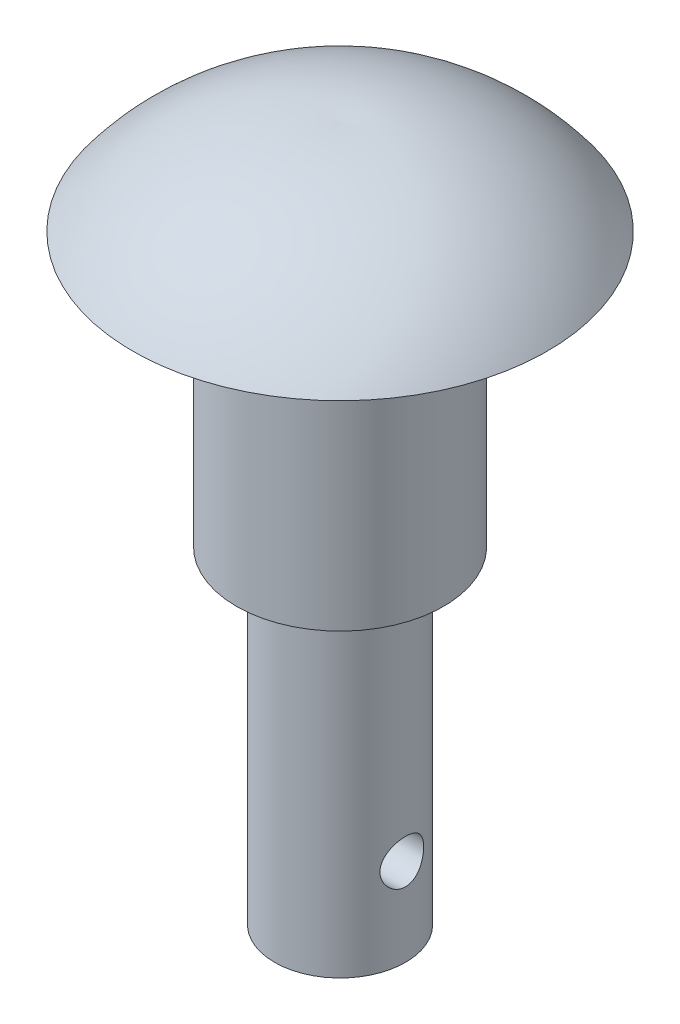
SolidWorks part; units mm, degrees
material "Plain Carbon Steel"
ref_plane "Front Plane" through (0, 0, 0) normal (0, 0, 1) x (1, 0, 0)
ref_plane "Top Plane" through (0, 0, 0) normal (0, 1, 0) x (1, 0, 0)
ref_plane "Right Plane" through (0, 0, 0) normal (1, 0, 0) x (0, 0, -1)
sketch "Shaft Profile Ø12" plane through (0, 0, 0) normal (0, 1, 0) x (1, 0, 0)
  circle A0 centre (0, 0) radius 6
  dimension "D1" = 12
extrude "Shaft Ø12" add sketch "Shaft Profile Ø12" along normal blind 30
sketch "Collar Profile Ø19" plane through (0, 30, 0) normal (0, 1, 0) x (1, 0, 0)
  circle A0 centre (0, 0) radius 9.5
  dimension "D1" = 19
extrude "Collar Ø19" add sketch "Collar Profile Ø19" along normal blind 25
sketch "Dome Head Profile" plane through (0, 0, 0) normal (1, 0, 0) x (0, 0, -1)
  line L0 (0, 55) -> (-19, 55)
  line L1 (9.5, 55) -> (-9.5, 55) construction
  line L2 (0, 55) -> (0, 63.7349)
  arc A0 (-19, 55) -> (0, 63.7349) centre (-1.4147, 41.7804) cw
  dimension "D1" = 22
  dimension "D2" = 1.4147
  dimension "D3" = 41.7804
revolve "Dome Head" add sketch "Dome Head Profile" angle 360 about L2
sketch "Cross Hole Profile" plane through (0, 0, 0) normal (1, 0, 0) x (0, 0, -1)
  line L0 (-6, 30) -> (6, 30) construction
  circle A0 centre (0, 8) radius 2
  dimension "D1" = 4
  dimension "D2" = 8
  dimension "D3" = 22
extrude "Cross Hole" cut sketch "Cross Hole Profile" against normal mid plane 25
